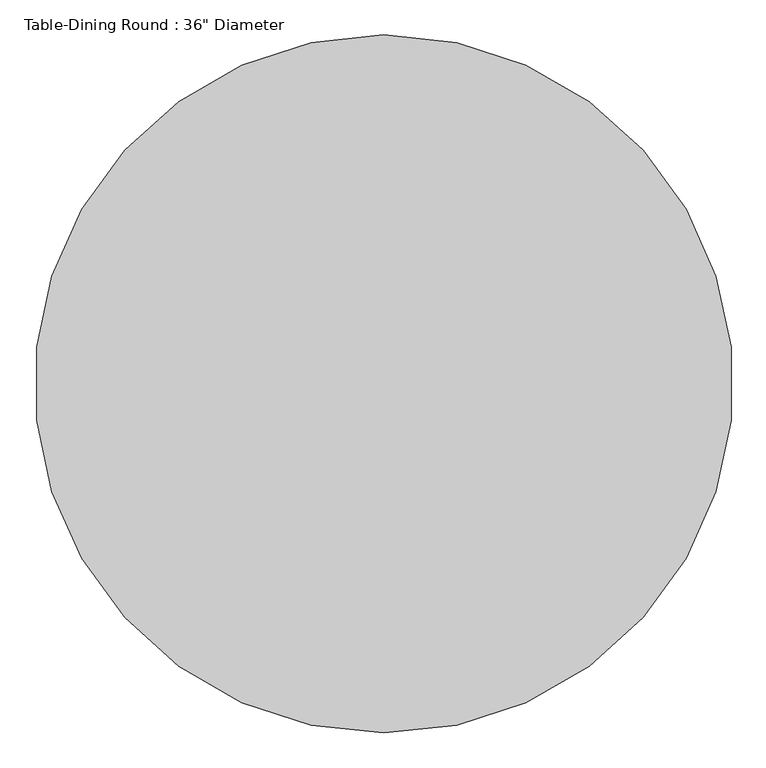
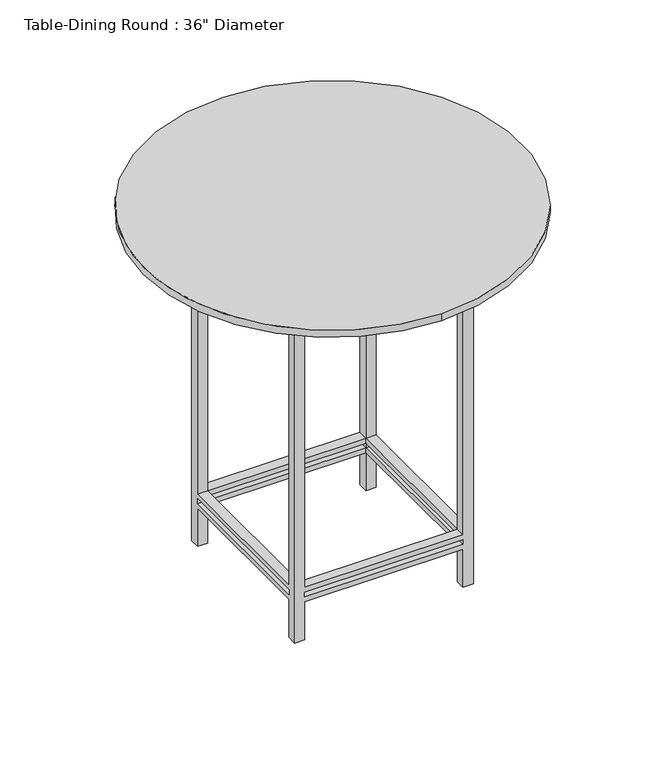
"""IFC4 building model written with IfcOpenShell, lengths in millimetres: furniture geometry."""

from ifc_helpers import new_model, si_unit, point, frame, frame_2d, origin, place, context, project, spatial, polyline, circle_curve, trimmed, segment, composite_curve, outline, extrude, faceted_brep, source, transform, mapped, element, save


def furniture_4371de90(model_context):
    return source(origin(), model_context, "Body", "SolidModel", [
        extrude(outline(polyline([(579.9319672, 291.3713115), (579.9319672, -661.1286885), (-372.5680328, -661.1286885), (-372.5680328, 291.3713115), (579.9319672, 291.3713115)]), holes=[polyline([(554.5319672, 265.9713115), (-347.1680328, 265.9713115), (-347.1680328, -635.7286885), (554.5319672, -635.7286885), (554.5319672, 265.9713115)])]), frame((0.0, 0.0, 1790.7), z_axis=(0.0, 0.0, 1.0), x_axis=(1.0, 0.0, 0.0)), (0.0, 0.0, 1.0), 76.2),
        faceted_brep([(-296.3680328, 265.9713115, 1866.9), (-347.1680328, 265.9713115, 1866.9), (-347.1680328, 215.1713115, 1866.9), (-296.3680328, 215.1713115, 1866.9), (503.7319672, 265.9713115, 1866.9), (503.7319672, 215.1713115, 1866.9), (554.5319672, 215.1713115, 1866.9), (554.5319672, 265.9713115, 1866.9), (503.7319672, -635.7286885, 1866.9), (554.5319672, -635.7286885, 1866.9), (554.5319672, -584.9286885, 1866.9), (503.7319672, -584.9286885, 1866.9), (-296.3680328, -635.7286885, 1866.9), (-296.3680328, -584.9286885, 1866.9), (-347.1680328, -584.9286885, 1866.9), (-347.1680328, -635.7286885, 1866.9), (-296.3680328, 265.9713115, 0.0), (-296.3680328, 215.1713115, 0.0), (-347.1680328, 215.1713115, 0.0), (-347.1680328, 265.9713115, 0.0), (503.7319672, 265.9713115, 0.0), (554.5319672, 265.9713115, 0.0), (554.5319672, 215.1713115, 0.0), (503.7319672, 215.1713115, 0.0), (503.7319672, -635.7286885, 0.0), (503.7319672, -584.9286885, 0.0), (554.5319672, -584.9286885, 0.0), (554.5319672, -635.7286885, 0.0), (-296.3680328, -635.7286885, 0.0), (-347.1680328, -635.7286885, 0.0), (-347.1680328, -584.9286885, 0.0), (-296.3680328, -584.9286885, 0.0), (-296.3680328, 265.9713115, 279.4), (503.7319672, 265.9713115, 279.4), (503.7319672, 265.9713115, 203.2), (-296.3680328, 265.9713115, 203.2), (503.7319672, 265.9713115, 228.6), (503.7319672, 265.9713115, 254.0), (-296.3680328, 265.9713115, 254.0), (-296.3680328, 265.9713115, 228.6), (-347.1680328, 215.1713115, 203.2), (-347.1680328, -584.9286885, 203.2), (-347.1680328, -584.9286885, 279.4), (-347.1680328, 215.1713115, 279.4), (-347.1680328, 215.1713115, 228.6), (-347.1680328, 215.1713115, 254.0), (-347.1680328, -584.9286885, 254.0), (-347.1680328, -584.9286885, 228.6), (-296.3680328, 215.1713115, 279.4), (-296.3680328, 215.1713115, 203.2), (-296.3680328, 215.1713115, 228.6), (-296.3680328, 215.1713115, 254.0), (503.7319672, 215.1713115, 279.4), (503.7319672, 215.1713115, 203.2), (503.7319672, 215.1713115, 228.6), (503.7319672, 215.1713115, 254.0), (554.5319672, 215.1713115, 279.4), (554.5319672, 215.1713115, 203.2), (554.5319672, 215.1713115, 228.6), (554.5319672, 215.1713115, 254.0), (554.5319672, -584.9286885, 279.4), (554.5319672, -584.9286885, 203.2), (554.5319672, -584.9286885, 228.6), (554.5319672, -584.9286885, 254.0), (503.7319672, -635.7286885, 279.4), (-296.3680328, -635.7286885, 279.4), (-296.3680328, -635.7286885, 203.2), (503.7319672, -635.7286885, 203.2), (-296.3680328, -635.7286885, 228.6), (-296.3680328, -635.7286885, 254.0), (503.7319672, -635.7286885, 254.0), (503.7319672, -635.7286885, 228.6), (503.7319672, -584.9286885, 279.4), (503.7319672, -584.9286885, 203.2), (503.7319672, -584.9286885, 228.6), (503.7319672, -584.9286885, 254.0), (-296.3680328, -584.9286885, 279.4), (-296.3680328, -584.9286885, 203.2), (-296.3680328, -584.9286885, 228.6), (-296.3680328, -584.9286885, 254.0)], [[[0, 1, 2, 3]], [[4, 5, 6, 7]], [[8, 9, 10, 11]], [[12, 13, 14, 15]], [[16, 17, 18, 19]], [[20, 21, 22, 23]], [[24, 25, 26, 27]], [[28, 29, 30, 31]], [[1, 0, 32, 33, 4, 7, 21, 20, 34, 35, 16, 19], [36, 37, 38, 39]], [[2, 1, 19, 18, 40, 41, 30, 29, 15, 14, 42, 43], [44, 45, 46, 47]], [[3, 2, 43, 48]], [[18, 17, 49, 40]], [[44, 50, 51, 45]], [[0, 3, 48, 32]], [[17, 16, 35, 49]], [[50, 39, 38, 51]], [[5, 4, 33, 52]], [[20, 23, 53, 34]], [[36, 54, 55, 37]], [[6, 5, 52, 56]], [[23, 22, 57, 53]], [[54, 58, 59, 55]], [[21, 7, 6, 56, 60, 10, 9, 27, 26, 61, 57, 22], [62, 63, 59, 58]], [[27, 9, 8, 64, 65, 12, 15, 29, 28, 66, 67, 24], [68, 69, 70, 71]], [[11, 10, 60, 72]], [[26, 25, 73, 61]], [[62, 74, 75, 63]], [[8, 11, 72, 64]], [[25, 24, 67, 73]], [[74, 71, 70, 75]], [[13, 12, 65, 76]], [[28, 31, 77, 66]], [[68, 78, 79, 69]], [[14, 13, 76, 42]], [[31, 30, 41, 77]], [[78, 47, 46, 79]], [[54, 74, 62, 58]], [[74, 78, 68, 71]], [[78, 50, 44, 47]], [[50, 54, 36, 39]], [[53, 49, 35, 34]], [[49, 77, 41, 40]], [[77, 73, 67, 66]], [[73, 53, 57, 61]], [[74, 54, 53, 73]], [[78, 74, 73, 77]], [[50, 78, 77, 49]], [[54, 50, 49, 53]], [[52, 72, 60, 56]], [[72, 76, 65, 64]], [[76, 48, 43, 42]], [[48, 52, 33, 32]], [[55, 51, 38, 37]], [[51, 79, 46, 45]], [[79, 75, 70, 69]], [[75, 55, 59, 63]], [[72, 52, 55, 75]], [[76, 72, 75, 79]], [[48, 76, 79, 51]], [[52, 48, 51, 55]]]),
        extrude(outline(composite_curve([segment(trimmed(circle_curve(frame_2d((103.6819672, -184.8786885)), 952.5), [point((103.6819672, -1137.3786885))], [point((103.6819672, 767.6213115))], False, "CARTESIAN"), True, "CONTINUOUS"), segment(trimmed(circle_curve(frame_2d((103.6819672, -184.8786885)), 952.5), [point((103.6819672, 767.6213115))], [point((103.6819672, -1137.3786885))], False, "CARTESIAN"), True, "CONTINUOUS")], self_intersect=False)), frame((0.0, 0.0, 1866.9), z_axis=(0.0, 0.0, 1.0), x_axis=(1.0, 0.0, 0.0)), (0.0, 0.0, 1.0), 38.1),
    ])


if __name__ == "__main__":
    model = new_model("IFC4")
    model_context = context("Model", 3, world=origin())
    ifc_project = project(units=[si_unit("LENGTHUNIT", "METRE", prefix="MILLI")], contexts=[model_context])
    site = spatial("IfcSite", under=ifc_project)
    building = spatial("IfcBuilding", under=site)
    placement = place(None, origin())
    furniture_shape = furniture_4371de90(model_context)
    element("IfcFurniture", 1, ObjectType="Table-Dining Round : 36\" Diameter", at=placement, inside=building, context=model_context, shape_type="MappedRepresentation", body=[
        mapped(furniture_shape, transform((0.0, 0.0, 0.0), x_axis=(1.0, 0.0, 0.0), y_axis=(0.0, 1.0, 0.0), z_axis=(0.0, 0.0, 1.0))),
    ])
    save(model, "model.ifc")

# Revit data of these elements
# Type "Table-Dining Round : 36\" Diameter"
#   Assembly Code = "E2020200"
#   Diameter = 6' - 3"
#   Height = 6' - 3"
#   Base Material = Pine
#   Top Material = Laminate, Linen, Matte
#   Default Elevation = 0
# Element 1 (IfcFurniture, "Table-Dining Round : 36\" Diameter")
#   Materials on its faces: "Pine", "Laminate, Linen, Matte"
# Materials
#   "Pine": class "Wood", colour RGB 223 192 134, transparency 0, Description = "Pinus Echinata", Cost = 0
#   "Laminate, Linen, Matte": class "Plastic", colour RGB 249 239 230, transparency 0, Description = "Plastic Laminate - Linen, Matte", Cost = 0
